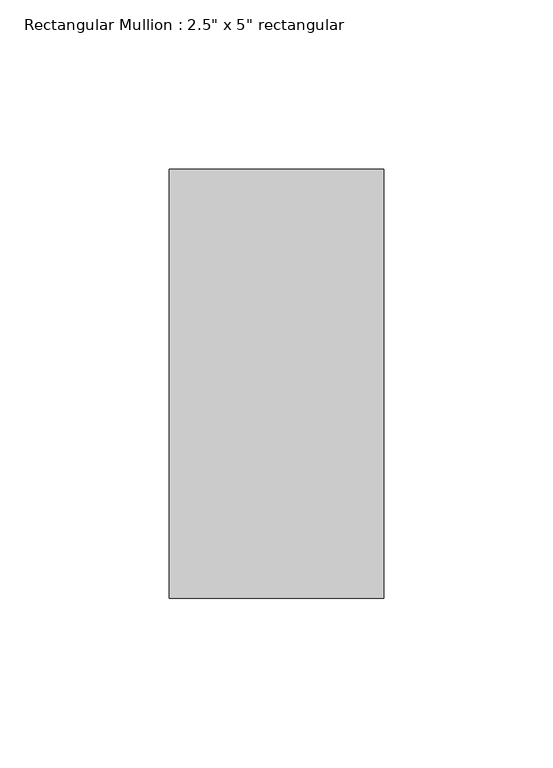
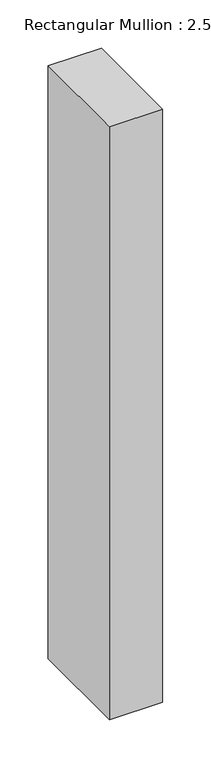
"""IFC4 building model written with IfcOpenShell, lengths in millimetres: member geometry."""

from ifc_helpers import new_model, si_unit, frame, origin, place, context, project, spatial, polyline, outline, extrude, source, transform, mapped, element, save


def member_b2e19614(model_context):
    return source(origin(), model_context, "Body", "SweptSolid", [
        extrude(outline(polyline([(31.75, 63.5), (31.75, -63.5), (-31.75, -63.5), (-31.75, 63.5), (31.75, 63.5)])), frame((0.0, 0.0, -748.4785678), z_axis=(0.0, 0.0, 1.0), x_axis=(1.0, 0.0, 0.0)), (0.0, 0.0, 1.0), 748.4785678),
    ])


if __name__ == "__main__":
    model = new_model("IFC4")
    model_context = context("Model", 3, world=origin())
    ifc_project = project(units=[si_unit("LENGTHUNIT", "METRE", prefix="MILLI")], contexts=[model_context])
    site = spatial("IfcSite", under=ifc_project)
    building = spatial("IfcBuilding", under=site)
    placement = place(None, origin())
    member_shape = member_b2e19614(model_context)
    element("IfcMember", 1, ObjectType="Rectangular Mullion : 2.5\" x 5\" rectangular", at=placement, inside=building, context=model_context, shape_type="MappedRepresentation", body=[
        mapped(member_shape, transform((0.0, 0.0, 0.0), x_axis=(1.0, 0.0, 0.0), y_axis=(0.0, 1.0, 0.0), z_axis=(0.0, 0.0, 1.0))),
    ])
    save(model, "model.ifc")

# Revit data of these elements
# Type "Rectangular Mullion : 2.5\" x 5\" rectangular"
#   built-in parameter 1007304 = 0.416667 (stored number, unit not read)
#   built-in parameter 1007301 = 0.104167 (stored number, unit not read)
#   built-in parameter 1007300 = 0.104167 (stored number, unit not read)
# Element 1 (IfcMember, "Rectangular Mullion : 2.5\" x 5\" rectangular")
#   Materials on its faces: "Aluminum"
# Materials
#   "Aluminum": class "Metal", colour RGB 247 247 247, transparency 0, Description = "Aluminum 6061", Cost = 0
